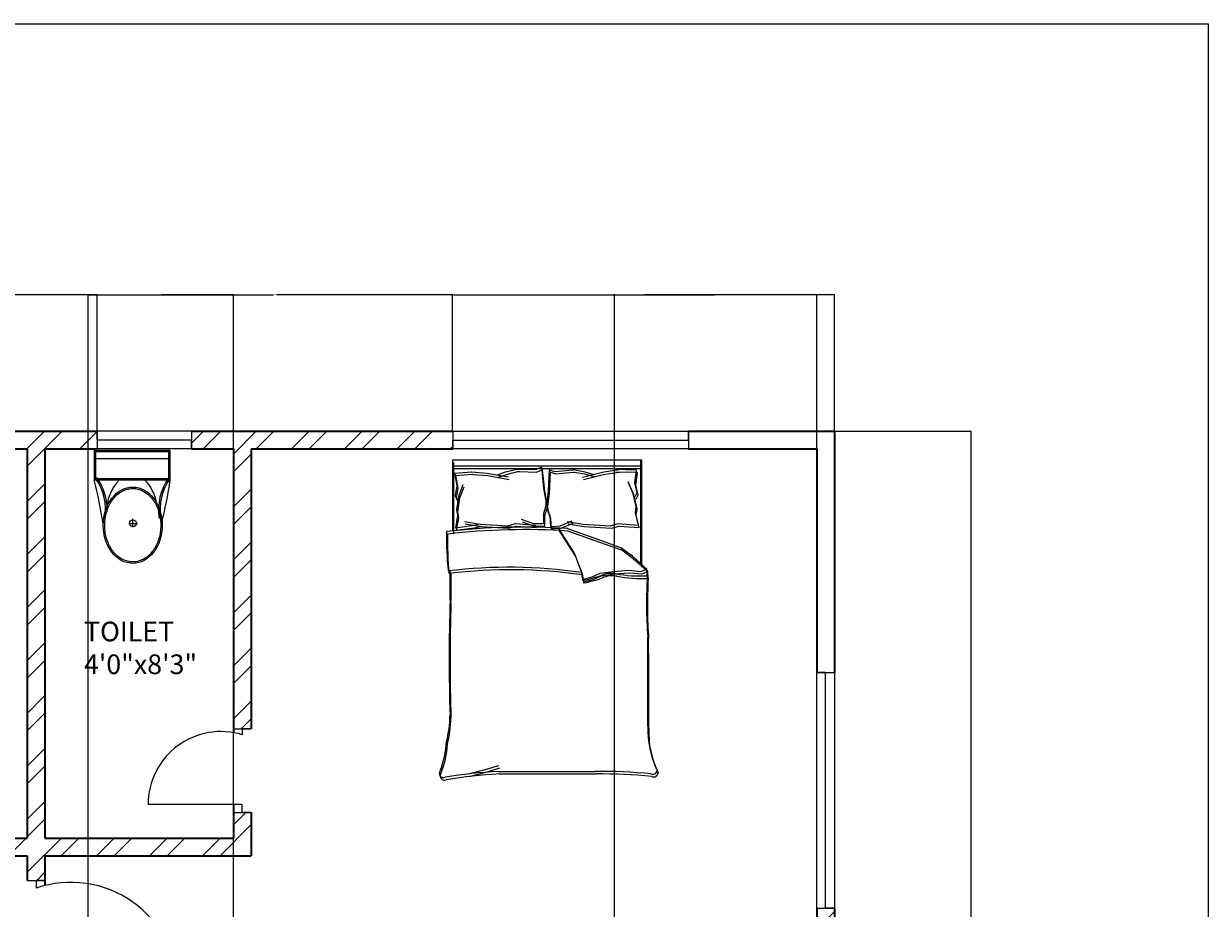
# Model space of a CAD drawing. Units: inches. Extents: x 1965 to 2673, y 1802 to 2669.
# Tile 16 of 16: x 2372 to 2673, y 2444 to 2669. Entities that reach past the tile are written whole.
import ezdxf

# ---------------------------------------------------------------- set-up
doc = ezdxf.new("R2010")
doc.units = ezdxf.units.IN
for name, color, linetype, lineweight in [('A-ANNO-DIMS', 2, 'Continuous', 18), ('A-ANNO-TTLB', 7, 'Continuous', 25), ('A-AREA-IDEN', 7, 'Continuous', 18), ('A-DOOR', 11, 'Continuous', 18), ('A-FLOR-FIXT', 9, 'Continuous', 18), ('A-FURN', 8, 'Continuous', 13), ('A-GLAZ', 181, 'Continuous', 18), ('A-WALL', 7, 'Continuous', 35), ('A-WALL-PATT', 252, 'Continuous', 13)]:
    doc.layers.add(name, color=color, linetype=linetype, lineweight=lineweight)
doc.styles.get("Standard").update_dxf_attribs({"font": 'arial.ttf'})
doc.dimstyles.get("Standard").update_dxf_attribs({"dimtxt": 0.18, "dimasz": 0.18, "dimexe": 0.18, "dimexo": 0.0625, "dimgap": 0.09, "dimtad": 0, "dimtih": 1, "dimtoh": 1, "dimdec": 4, "dimzin": 0, "dimdsep": 46, "dimtxsty": 'Standard', "dimcen": 0.09, "dimadec": 0, "dimazin": 0, "dimtfac": 1, "dimtdec": 4, "dimtofl": 0, "dimtmove": 0, "dimatfit": 3, "dimfxl": 1, "dimtolj": 1, "dimtzin": 0, "dimarcsym": 0})

# ---------------------------------------------------------------- blocks, each defined once
blk = doc.blocks.new('A$C31115884')
for p, q in [((283.1, 497.7), (223.4, 497.7)), ((257.5, 466.4), (257.5, 523.2)), ((0, 200), (0, 0)), ((520, 200), (0, 200)), ((10, 190), (10, 10)), ((510, 190), (10, 190)), ((510, 10), (510, 190)), ((520, 0), (520, 200)), ((510, 54.5), (0, 54.5)), ((10, 10), (510, 10)), ((0, 0), (520, 0))]:
    blk.add_line(p, q)
blk.add_circle((255.6, 496.4), 23.6)
for centre, radius, start, end in [((2777.7, -204.6), 2807, 165.4549, 171.71327), ((3237, 905), 2807, 188.28673, 194.5451), ((-294.5, 403.3), 364.7, 324.20913, 9.34987), ((-294.5, 403.3), 374.7, 324.20913, 9.34987), ((139.5, 406.2), 293.5, 315.84364, 2.65635), ((805.8, 403.3), 374.7, 179.20365, 215.79087), ((805.8, 403.3), 364.7, 170.65013, 215.79087), ((383.6, 406.2), 293.5, 190.27735, 224.15636)]:
    blk.add_arc(centre, radius, start, end)
blk.add_ellipse((256.2, 509.9), major_axis=(0, -260.7), ratio=0.772727)
blk.add_open_spline([(256.2, 259.2), (263.1, 259.2), (270, 259.7), (287.8, 262.3), (298.7, 265.1), (319.9, 273.1), (330.2, 278.4), (350.1, 291.1), (359.7, 298.7), (377.7, 315.9), (386.2, 325.5), (401.7, 346.6), (408.8, 358.1), (421.3, 382.5), (426.8, 395.5), (435.9, 422.4), (439.5, 436.4), (444.8, 465.1), (446.5, 479.7), (447.9, 509.2), (447.6, 524), (445, 553.3), (442.7, 567.8), (436.3, 596), (432.1, 609.7), (421.9, 636), (416, 648.6), (402.5, 672.1), (395, 683), (378.6, 703), (369.8, 712.1), (351.1, 728), (341.3, 734.8), (320.9, 746.2), (310.4, 750.7), (288.9, 757.3), (278, 759.4), (256, 761), (245, 760.6), (223.1, 757.2), (212.3, 754.3), (191.1, 746.1), (180.8, 740.7), (160.9, 727.8), (151.4, 720.1), (133.5, 702.7), (125.1, 693), (109.6, 671.7), (102.6, 660.2), (90.2, 635.7), (84.9, 622.7), (76, 595.6), (72.4, 581.6), (67.2, 552.9), (65.6, 538.2), (64.4, 508.8), (64.8, 494), (67.5, 464.7), (69.9, 450.2), (76.6, 422), (80.8, 408.3), (91.1, 382.2), (97.2, 369.7), (110.8, 346.3), (118.4, 335.4), (134.8, 315.6), (143.7, 306.7), (162.4, 290.9), (172.3, 284.2), (192.8, 273), (203.3, 268.6), (224.8, 262.2), (235.8, 260.2), (249.9, 259.3), (253, 259.2), (256.2, 259.2)], degree=3, knots=[0, 0, 0, 0, 0.110105, 0.110105, 0.285049, 0.285049, 0.459994, 0.459994, 0.634938, 0.634938, 0.809882, 0.809882, 0.984827, 0.984827, 1.159771, 1.159771, 1.334715, 1.334715, 1.50966, 1.50966, 1.684604, 1.684604, 1.859549, 1.859549, 2.034493, 2.034493, 2.209437, 2.209437, 2.384382, 2.384382, 2.559326, 2.559326, 2.73427, 2.73427, 2.909215, 2.909215, 3.084159, 3.084159, 3.259103, 3.259103, 3.434048, 3.434048, 3.608992, 3.608992, 3.783936, 3.783936, 3.958881, 3.958881, 4.133825, 4.133825, 4.30877, 4.30877, 4.483714, 4.483714, 4.658658, 4.658658, 4.833603, 4.833603, 5.008547, 5.008547, 5.183491, 5.183491, 5.358436, 5.358436, 5.53338, 5.53338, 5.708324, 5.708324, 5.883269, 5.883269, 6.058213, 6.058213, 6.233158, 6.233158, 6.283185, 6.283185, 6.283185, 6.283185])
blk = doc.blocks.new('BED-DOUBLE')
for p, q in [((3.47, 63.33), (3.47, 81.44)), ((3.47, 63.33), (3.47, 81.44)), ((3.47, 81.44), (51.49, 81.44)), ((51.26, 81.44), (51.26, 54.83)), ((51.26, 81.44), (51.26, 54.83)), ((51.49, 81.44), (51.49, 80.8)), ((3.47, 79.91), (51.26, 79.91)), ((3.47, 79.91), (51.26, 79.91)), ((3.7, 62.69), (3.7, 80.8)), ((3.7, 62.69), (3.7, 80.8)), ((3.7, 79.27), (51.49, 79.27)), ((3.7, 79.27), (51.49, 79.27)), ((3.89, 78.1), (8.17, 78.43)), ((3.89, 78.1), (8.17, 78.43)), ((8.17, 78.43), (8.28, 78.41)), ((8.17, 78.43), (8.28, 78.41)), ((8.28, 78.41), (12.1, 78.12)), ((8.28, 78.41), (12.1, 78.12)), ((14.85, 77.69), (16.87, 78.41)), ((14.85, 77.69), (16.87, 78.41)), ((16.87, 78.41), (19.76, 79.14)), ((16.87, 78.41), (19.76, 79.14)), ((17.1, 77.77), (19.99, 78.5)), ((17.1, 77.77), (19.99, 78.5)), ((19.76, 79.14), (20.09, 79.14)), ((19.76, 79.14), (20.09, 79.14)), ((19.99, 78.5), (20.31, 78.5)), ((19.99, 78.5), (20.31, 78.5)), ((20.09, 79.14), (24.53, 78.99)), ((20.09, 79.14), (24.53, 78.99)), ((20.31, 78.5), (24.76, 78.35)), ((20.31, 78.5), (24.76, 78.35)), ((24.53, 78.99), (25.98, 79.57)), ((24.53, 78.99), (25.98, 79.57)), ((24.76, 78.35), (26.21, 78.93)), ((24.76, 78.35), (26.21, 78.93)), ((25.98, 79.57), (26.56, 74.22)), ((25.98, 79.57), (26.56, 74.22)), ((26.21, 78.93), (26.78, 73.58)), ((26.21, 78.93), (26.78, 73.58)), ((27.97, 78.95), (27.73, 73.57)), ((27.97, 78.95), (27.73, 73.57)), ((29.45, 78.46), (27.97, 78.95)), ((29.45, 78.46), (27.97, 78.95)), ((33.88, 78.88), (29.45, 78.46)), ((33.88, 78.88), (29.45, 78.46)), ((34.2, 78.9), (33.88, 78.88)), ((34.2, 78.9), (33.88, 78.88)), ((37.13, 78.36), (34.2, 78.9)), ((37.13, 78.36), (34.2, 78.9)), ((45.71, 78.9), (41.91, 78.37)), ((45.71, 78.9), (41.91, 78.37)), ((50.11, 78.88), (44.7, 78.98)), ((44.7, 78.98), (45.71, 78.9)), ((50.11, 78.88), (44.7, 78.98)), ((44.7, 78.98), (45.71, 78.9)), ((50.11, 78.88), (49.73, 75.67)), ((50.11, 78.88), (49.73, 75.67)), ((51.49, 80.8), (51.49, 54.19)), ((51.49, 80.8), (51.49, 54.19)), ((3.89, 78.12), (4.47, 74.94)), ((3.89, 78.12), (4.47, 74.94)), ((4.12, 77.46), (8.4, 77.79)), ((4.12, 77.46), (8.4, 77.79)), ((4.12, 77.49), (4.7, 74.3)), ((4.12, 77.49), (4.7, 74.3)), ((8.4, 77.79), (8.51, 77.77)), ((8.4, 77.79), (8.51, 77.77)), ((8.51, 77.77), (12.33, 77.49)), ((8.51, 77.77), (12.33, 77.49)), ((12.1, 78.12), (17.6, 77.11)), ((12.1, 78.12), (17.6, 77.11)), ((12.33, 77.49), (17.82, 76.47)), ((12.33, 77.49), (17.82, 76.47)), ((15.08, 77.05), (17.1, 77.77)), ((15.08, 77.05), (17.1, 77.77)), ((28.2, 78.31), (27.96, 72.93)), ((28.2, 78.31), (27.96, 72.93)), ((29.68, 77.82), (28.2, 78.31)), ((29.68, 77.82), (28.2, 78.31)), ((34.11, 78.24), (29.68, 77.82)), ((34.11, 78.24), (29.68, 77.82)), ((34.43, 78.26), (34.11, 78.24)), ((34.43, 78.26), (34.11, 78.24)), ((37.36, 77.72), (34.43, 78.26)), ((37.36, 77.72), (34.43, 78.26)), ((41.91, 78.37), (36.49, 77.02)), ((41.91, 78.37), (36.49, 77.02)), ((42.14, 77.73), (36.72, 76.38)), ((42.14, 77.73), (36.72, 76.38)), ((39.2, 77.77), (37.13, 78.36)), ((39.19, 77.77), (37.13, 78.36)), ((39.42, 77.13), (37.36, 77.72)), ((39.42, 77.13), (37.36, 77.72)), ((45.94, 78.26), (42.14, 77.73)), ((45.94, 78.26), (42.14, 77.73)), ((50.34, 78.24), (44.93, 78.34)), ((44.93, 78.34), (45.94, 78.26)), ((50.34, 78.24), (44.93, 78.34)), ((44.93, 78.34), (45.94, 78.26)), ((49.3, 73.18), (48.12, 75.86)), ((49.3, 73.18), (48.12, 75.86)), ((49.73, 75.67), (50.32, 73.1)), ((49.73, 75.67), (50.32, 73.1)), ((50.34, 78.24), (49.96, 75.03)), ((50.34, 78.24), (49.96, 75.03)), ((4.47, 74.94), (4.03, 72.34)), ((4.47, 74.94), (4.03, 72.34)), ((4.7, 74.3), (4.26, 71.7)), ((4.7, 74.3), (4.26, 71.7)), ((4.47, 68.87), (5.05, 72.49)), ((4.47, 68.87), (5.05, 72.49)), ((5.05, 72.49), (6.06, 75.23)), ((5.05, 72.49), (6.06, 75.23)), ((5.27, 71.85), (6.29, 74.59)), ((5.27, 71.85), (6.29, 74.59)), ((26.56, 74.22), (27.13, 71.04)), ((26.56, 74.22), (27.13, 71.04)), ((26.78, 73.58), (27.36, 70.4)), ((26.78, 73.58), (27.36, 70.4)), ((27.73, 73.57), (27.35, 70.36)), ((27.73, 73.57), (27.35, 70.36)), ((27.96, 72.93), (27.58, 69.72)), ((27.96, 72.93), (27.58, 69.72)), ((49.53, 72.54), (48.35, 75.22)), ((49.53, 72.54), (48.35, 75.22)), ((50.11, 69.61), (49.3, 73.18)), ((50.11, 69.61), (49.3, 73.18)), ((50.34, 68.97), (49.53, 72.54)), ((50.34, 68.97), (49.53, 72.54)), ((50.32, 73.1), (49.81, 72.06)), ((50.32, 73.1), (49.81, 72.06)), ((49.96, 75.03), (50.55, 72.46)), ((49.96, 75.03), (50.55, 72.46)), ((50.55, 72.46), (50.04, 71.42)), ((50.55, 72.46), (50.04, 71.42)), ((4.03, 72.34), (4.61, 71.33)), ((4.03, 72.34), (4.61, 71.33)), ((4.26, 71.7), (4.84, 70.69)), ((4.26, 71.7), (4.84, 70.69)), ((4.7, 68.23), (5.27, 71.85)), ((4.7, 68.23), (5.27, 71.85)), ((27.13, 69.74), (26.56, 67.86)), ((27.13, 69.74), (26.56, 67.86)), ((27.13, 71.04), (27.13, 69.74)), ((27.13, 71.04), (27.13, 69.74)), ((27.35, 70.36), (27.43, 69.06)), ((27.35, 70.36), (27.43, 69.06)), ((27.36, 70.4), (27.36, 69.1)), ((27.36, 70.4), (27.36, 69.1)), ((27.58, 69.72), (27.66, 68.42)), ((27.58, 69.72), (27.66, 68.42)), ((49.92, 68.01), (50.11, 69.61)), ((49.92, 68.01), (50.11, 69.61)), ((4.18, 64.1), (4.76, 67.28)), ((4.18, 64.1), (4.76, 67.28)), ((4.41, 63.46), (4.99, 66.64)), ((4.41, 63.46), (4.99, 66.64)), ((4.76, 67.28), (4.47, 68.87)), ((4.76, 67.28), (4.47, 68.87)), ((4.99, 66.64), (4.7, 68.23)), ((4.99, 66.64), (4.7, 68.23)), ((26.56, 67.86), (26.56, 65.18)), ((26.56, 67.86), (26.56, 65.18)), ((27.36, 69.1), (26.78, 67.22)), ((27.36, 69.1), (26.78, 67.22)), ((26.78, 67.22), (26.78, 64.54)), ((26.78, 67.22), (26.78, 64.54)), ((27.43, 69.06), (28.13, 67.22)), ((27.43, 69.06), (28.13, 67.22)), ((27.66, 68.42), (28.35, 66.58)), ((27.66, 68.42), (28.35, 66.58)), ((28.13, 67.22), (28.29, 64.55)), ((28.13, 67.22), (28.29, 64.55)), ((28.35, 66.58), (28.52, 63.91)), ((28.35, 66.58), (28.52, 63.91)), ((50.69, 64.87), (49.92, 68.01)), ((50.69, 64.87), (49.92, 68.01)), ((50.15, 67.37), (50.34, 68.97)), ((50.15, 67.37), (50.34, 68.97)), ((50.92, 64.23), (50.15, 67.37)), ((50.92, 64.23), (50.15, 67.37)), ((9.28, 64.82), (4.18, 64.1)), ((9.28, 64.82), (4.18, 64.1)), ((9.5, 64.18), (4.41, 63.46)), ((9.5, 64.18), (4.41, 63.46)), ((6.38, 65.81), (10.41, 65.15)), ((6.38, 65.81), (10.41, 65.15)), ((6.6, 65.17), (10.64, 64.51)), ((6.61, 65.17), (10.64, 64.51)), ((10.41, 65.15), (9.28, 64.82)), ((10.41, 65.15), (9.28, 64.82)), ((10.64, 64.51), (9.5, 64.18)), ((10.64, 64.51), (9.5, 64.18)), ((10.41, 65.15), (17.42, 64.71)), ((10.41, 65.15), (17.42, 64.71)), ((10.64, 64.51), (17.65, 64.08)), ((10.64, 64.51), (17.65, 64.08)), ((17.42, 64.71), (19.38, 65.27)), ((17.42, 64.71), (19.38, 65.27)), ((17.65, 64.08), (19.61, 64.63)), ((17.65, 64.08), (19.61, 64.63)), ((19.38, 65.27), (24.51, 64.87)), ((19.38, 65.27), (24.51, 64.87)), ((19.61, 64.63), (24.74, 64.23)), ((19.61, 64.63), (24.74, 64.23)), ((24.1, 65.18), (20.95, 66.27)), ((24.1, 65.18), (20.95, 66.27)), ((24.33, 64.54), (21.18, 65.63)), ((24.33, 64.54), (21.18, 65.63)), ((26.56, 65.18), (24.1, 65.18)), ((26.56, 65.18), (24.1, 65.18)), ((26.78, 64.54), (24.33, 64.54)), ((26.78, 64.54), (24.33, 64.54)), ((28.29, 64.55), (30.75, 64.7)), ((28.29, 64.55), (30.75, 64.7)), ((28.52, 63.91), (30.97, 64.06)), ((28.52, 63.91), (30.97, 64.06)), ((30.25, 64.06), (34.44, 57.56)), ((30.25, 64.06), (34.44, 57.56)), ((30.48, 63.42), (34.67, 56.92)), ((30.48, 63.42), (34.67, 56.92)), ((30.75, 64.7), (33.82, 65.99)), ((30.75, 64.7), (33.82, 65.99)), ((30.97, 64.06), (34.04, 65.35)), ((30.97, 64.06), (34.04, 65.35)), ((40.64, 61.12), (32.3, 64.06)), ((40.64, 61.12), (32.3, 64.06)), ((40.87, 60.48), (32.53, 63.42)), ((40.87, 60.48), (32.53, 63.42)), ((32.56, 65.81), (36.59, 65.15)), ((32.56, 65.81), (36.59, 65.15)), ((32.79, 65.17), (36.82, 64.51)), ((32.79, 65.17), (36.82, 64.51)), ((36.59, 65.15), (43.6, 64.71)), ((36.59, 65.15), (43.6, 64.71)), ((36.82, 64.51), (43.83, 64.08)), ((36.82, 64.51), (43.83, 64.08)), ((43.6, 64.71), (45.56, 65.27)), ((43.6, 64.71), (45.56, 65.27)), ((43.83, 64.08), (45.79, 64.63)), ((43.83, 64.08), (45.79, 64.63)), ((45.56, 65.27), (50.69, 64.87)), ((45.56, 65.27), (50.69, 64.87)), ((45.79, 64.63), (50.92, 64.23)), ((45.79, 64.63), (50.92, 64.23)), ((46.21, 59.11), (40.64, 61.12)), ((46.21, 59.11), (40.64, 61.12)), ((46.44, 58.47), (40.87, 60.48)), ((46.44, 58.47), (40.87, 60.48)), ((34.44, 57.56), (36.15, 53.08)), ((34.44, 57.56), (36.15, 53.08)), ((49.16, 56.95), (46.21, 59.11)), ((49.16, 56.95), (46.21, 59.11)), ((49.39, 56.31), (46.44, 58.47)), ((49.39, 56.31), (46.44, 58.47)), ((34.67, 56.92), (36.38, 52.44)), ((34.67, 56.92), (36.38, 52.44)), ((52.86, 53.69), (49.16, 56.95)), ((52.86, 53.69), (49.16, 56.95)), ((53.09, 53.06), (49.39, 56.31)), ((53.09, 53.06), (49.39, 56.31)), ((36.15, 53.08), (36.46, 51.06)), ((36.15, 53.08), (36.46, 51.06)), ((36.38, 52.44), (36.69, 50.42)), ((36.38, 52.44), (36.69, 50.42)), ((36.46, 51.06), (38.94, 51.68)), ((36.46, 51.06), (38.94, 51.68)), ((38.94, 51.68), (40.95, 52.61)), ((38.94, 51.68), (40.95, 52.61)), ((39.16, 51.04), (41.18, 51.97)), ((39.16, 51.04), (41.18, 51.97)), ((40.95, 52.61), (44.36, 53.08)), ((40.95, 52.61), (44.36, 53.08)), ((41.18, 51.97), (44.58, 52.44)), ((41.18, 51.97), (44.58, 52.44)), ((44.36, 53.08), (48.23, 53.39)), ((44.36, 53.08), (48.23, 53.39)), ((44.58, 52.44), (48.46, 52.75)), ((44.58, 52.44), (48.46, 52.75)), ((48.23, 53.39), (51.33, 53.08)), ((48.23, 53.39), (51.33, 53.08)), ((48.46, 52.75), (51.55, 52.44)), ((48.46, 52.75), (51.55, 52.44)), ((51.33, 53.08), (52.86, 53.69)), ((51.33, 53.08), (52.86, 53.69)), ((51.55, 52.44), (53.09, 53.06)), ((51.55, 52.44), (53.09, 53.06)), ((52.94, 51.95), (52.86, 53.69, 3.87)), ((52.94, 51.95), (52.86, 53.69, 3.87)), ((53.17, 51.31), (53.09, 53.06, 3.87)), ((53.17, 51.31), (53.09, 53.06, 3.87)), ((36.69, 50.42), (39.16, 51.04)), ((36.69, 50.42), (39.16, 51.04)), ((15.06, 2.2), (39.67, 2.2)), ((15.06, 2.2), (39.67, 2.2)), ((15.29, 1.56), (39.9, 1.56)), ((15.29, 1.56), (39.9, 1.56))]:
    blk.add_line(p, q)
for centre, radius, start, end in [((21.35, -100.61), 164.97, 86.0865, 96.7821), ((21.35, -100.61), 164.97, 86.0865, 96.7821), ((21.58, -101.25), 164.97, 86.0865, 96.7821), ((21.58, -101.25), 164.97, 86.0865, 96.7821), ((85.16, 61.34), 83.31, 178.7218, 185.604), ((85.16, 61.34), 83.31, 178.7218, 185.604), ((85.39, 60.71), 83.31, 178.7218, 185.604), ((85.38, 60.71), 83.31, 178.7218, 185.604), ((17.75, -74.88), 129.02, 81.7845, 96.9006), ((17.75, -74.88), 129.02, 81.7845, 96.9006), ((17.98, -75.51), 129.02, 81.7845, 96.9006), ((17.98, -75.51), 129.02, 81.7845, 96.9006), ((-167.31, 50.27), 170.11, 358.4762, 1.0082), ((-167.31, 50.27), 170.11, 358.4762, 1.0082), ((-167.08, 49.63), 170.11, 358.4762, 1.0082), ((-167.08, 49.63), 170.11, 358.4762, 1.0082), ((31.15, 79.96), 29.65, 280.6617, 289.8806), ((31.15, 79.96), 29.65, 280.6617, 289.8806), ((31.38, 79.32), 29.65, 280.6617, 289.8806), ((31.38, 79.32), 29.65, 280.6617, 289.8806), ((43.74, 46.37), 6.22, 78.6608, 113.7384), ((43.74, 46.37), 6.22, 78.6608, 113.7384), ((43.97, 45.74), 6.22, 78.6608, 113.7384), ((43.97, 45.74), 6.22, 78.6608, 113.7384), ((51.32, 88.1), 36.18, 259.8763, 272.5657), ((51.32, 88.1), 36.18, 259.8763, 272.5657), ((51.55, 87.46), 36.18, 259.8763, 272.5657), ((51.55, 87.46), 36.18, 259.8763, 272.5657), ((182.26, 45.13), 129.5, 176.9791, 183.8365), ((182.26, 45.13), 129.5, 176.9791, 183.8365), ((182.49, 44.49), 129.5, 176.9791, 183.8365), ((182.49, 44.49), 129.5, 176.9791, 183.8365), ((36.63, 51), 0.185, 160.2464, 271.1377), ((36.63, 51), 0.185, 160.2464, 271.1377), ((36.86, 50.36), 0.185, 160.2464, 271.1377), ((36.86, 50.36), 0.185, 160.2464, 271.1377), ((484.82, 30.83), 482.31, 178.2277, 181.7185), ((484.82, 30.83), 482.31, 178.2277, 181.7185), ((485.05, 30.19), 482.31, 178.2277, 181.7185), ((485.05, 30.19), 482.31, 178.2277, 181.7185), ((-4508.75, 13.62), 4561.86, 0.00217, 0.28689), ((-4508.75, 13.62), 4561.86, 0.00217, 0.28689), ((-4508.52, 12.98), 4561.86, 0.00217, 0.28689), ((-4508.52, 12.98), 4561.86, 0.00217, 0.28689), ((-26.9, 16.93), 29.63, 346.0648, 358.9113), ((-26.9, 16.93), 29.63, 346.0648, 358.9113), ((-26.68, 16.29), 29.63, 346.0648, 358.9113), ((-26.68, 16.29), 29.63, 346.0648, 358.9113), ((76.15, 12.77), 23.07, 177.4714, 206.4681), ((76.15, 12.77), 23.07, 177.4714, 206.4681), ((76.38, 12.14), 23.07, 177.4714, 206.4681), ((76.38, 12.14), 23.07, 177.4714, 206.4681), ((-21.66, 11.17), 23.56, 337.9751, 356.652), ((-21.66, 11.17), 23.56, 337.9751, 356.652), ((-21.44, 10.53), 23.56, 337.9751, 356.652), ((-21.44, 10.53), 23.56, 337.9751, 356.652), ((-17.23, 105.15), 106.46, 283.3832, 287.7053), ((-17.23, 105.15), 106.46, 283.3832, 287.7053), ((-17, 104.51), 106.46, 283.3832, 287.7053), ((-17, 104.51), 106.46, 283.3832, 287.7053), ((1.08, 1.72), 1.09, 146.1736, 293.4781), ((1.08, 1.72), 1.09, 146.1736, 293.4781), ((1.31, 1.08), 1.09, 146.1736, 293.4781), ((1.31, 1.08), 1.09, 146.1736, 293.4781), ((21.42, -119.4), 121.76, 92.9958, 99.4091), ((21.42, -119.4), 121.76, 92.9958, 99.4091), ((21.65, -120.04), 121.76, 92.9958, 99.4091), ((21.65, -120.04), 121.76, 92.9958, 99.4091), ((41.15, -130.84), 133.04, 84.4998, 90.6351), ((41.15, -130.84), 133.04, 84.4998, 90.6351), ((41.38, -131.48), 133.04, 84.4998, 90.6351), ((41.37, -131.48), 133.04, 84.4998, 90.6351), ((54.4, 2.57), 1.1, 242.6588, 356.02), ((54.4, 2.57), 1.1, 242.6588, 356.02), ((54.63, 1.93), 1.1, 242.6588, 356.02), ((54.63, 1.93), 1.1, 242.6588, 356.02)]:
    blk.add_arc(centre, radius, start, end)
blk = doc.blocks.new('WIN-60IN')
for p, q in [((0, 4.5), (0, 0)), ((0, 4.5), (60, 4.5)), ((60, 2.25), (60, 4.5)), ((60, 4.5), (60, 0)), ((0, 0), (0, 2.25)), ((0, 2.25), (60, 2.25)), ((60, 0), (0, 0))]:
    blk.add_line(p, q)
blk = doc.blocks.new('WIN-24IN')
for p, q in [((0, 24), (4.5, 24)), ((0, 24), (0, 0)), ((4.5, 24), (2.25, 24)), ((2.25, 24), (2.25, 0)), ((4.5, 24), (4.5, 0)), ((2.25, 0), (0, 0)), ((0, 0), (4.5, 0))]:
    blk.add_line(p, q)
blk = doc.blocks.new('*D26')
at = {"layer": 'A-ANNO-DIMS', "color": 0, "lineweight": -2, "transparency": 16777216}
for p, q in [((2578.16, 2565.59), (2613, 2565.59)), ((2612.82, 2565.41), (2612.82, 2248.77)), ((2612.82, 1931.77), (2612.82, 2248.41)), ((2578.16, 1931.59), (2613, 1931.59))]:
    blk.add_line(p, q, dxfattribs=at)
at = {"layer": 'A-ANNO-DIMS', "color": 0, "transparency": 16777216}
for points in [[(2612.79, 2565.41), (2612.85, 2565.41), (2612.82, 2565.59)], [(2612.79, 1931.77), (2612.85, 1931.77), (2612.82, 1931.59)]]:
    blk.add_solid(points, dxfattribs=at)
at = {"layer": 'Defpoints', "color": 0, "transparency": 16777216}
for p in [(2578.09, 2565.59), (2612.82, 2565.59), (2578.09, 1931.59)]:
    blk.add_point(p, dxfattribs=at)
at = {"layer": 'A-ANNO-DIMS', "color": 0, "transparency": 16777216, "insert": (2612.82, 2248.59), "char_height": 0.18, "attachment_point": 5}
blk.add_mtext('\\A1;634', dxfattribs=at)
blk = doc.blocks.new('*D30')
at = {"layer": 'A-ANNO-DIMS', "color": 0, "lineweight": -2, "transparency": 16777216}
for p, q in [((2285.97, 2565.65), (2285.97, 2600.5)), ((2286.15, 2600.32), (2337.74, 2600.32)), ((2390.24, 2600.32), (2338.65, 2600.32)), ((2390.42, 2565.65), (2390.42, 2600.5))]:
    blk.add_line(p, q, dxfattribs=at)
at = {"layer": 'A-ANNO-DIMS', "color": 0, "transparency": 16777216}
for points in [[(2286.15, 2600.35), (2286.15, 2600.29), (2285.97, 2600.32)], [(2390.24, 2600.35), (2390.24, 2600.29), (2390.42, 2600.32)]]:
    blk.add_solid(points, dxfattribs=at)
at = {"layer": 'Defpoints', "color": 0, "transparency": 16777216}
for p in [(2390.42, 2600.32), (2285.97, 2565.59), (2390.42, 2565.59)]:
    blk.add_point(p, dxfattribs=at)
at = {"layer": 'A-ANNO-DIMS', "color": 0, "transparency": 16777216, "insert": (2338.2, 2600.32), "char_height": 0.18, "attachment_point": 5}
blk.add_mtext('\\A1;104.44', dxfattribs=at)
blk = doc.blocks.new('*D31')
at = {"layer": 'A-ANNO-DIMS', "color": 0, "lineweight": -2, "transparency": 16777216}
for p, q in [((2390.42, 2565.65), (2390.42, 2600.5)), ((2390.6, 2600.32), (2435.26, 2600.32)), ((2480.71, 2600.32), (2436.05, 2600.32)), ((2480.89, 2565.65), (2480.89, 2600.5))]:
    blk.add_line(p, q, dxfattribs=at)
at = {"layer": 'A-ANNO-DIMS', "color": 0, "transparency": 16777216}
for points in [[(2390.6, 2600.35), (2390.6, 2600.29), (2390.42, 2600.32)], [(2480.71, 2600.35), (2480.71, 2600.29), (2480.89, 2600.32)]]:
    blk.add_solid(points, dxfattribs=at)
at = {"layer": 'Defpoints', "color": 0, "transparency": 16777216}
for p in [(2480.89, 2600.32), (2390.42, 2565.59), (2480.89, 2565.59)]:
    blk.add_point(p, dxfattribs=at)
at = {"layer": 'A-ANNO-DIMS', "color": 0, "transparency": 16777216, "insert": (2435.66, 2600.32), "char_height": 0.18, "attachment_point": 5}
blk.add_mtext('\\A1;90.48', dxfattribs=at)
blk = doc.blocks.new('*D32')
at = {"layer": 'A-ANNO-DIMS', "color": 0, "lineweight": -2, "transparency": 16777216}
for p, q in [((2480.89, 2565.65), (2480.89, 2600.5)), ((2481.07, 2600.32), (2529.17, 2600.32)), ((2577.91, 2600.32), (2529.82, 2600.32)), ((2578.09, 2565.65), (2578.09, 2600.5))]:
    blk.add_line(p, q, dxfattribs=at)
at = {"layer": 'A-ANNO-DIMS', "color": 0, "transparency": 16777216}
for points in [[(2481.07, 2600.35), (2481.07, 2600.29), (2480.89, 2600.32)], [(2577.91, 2600.35), (2577.91, 2600.29), (2578.09, 2600.32)]]:
    blk.add_solid(points, dxfattribs=at)
at = {"layer": 'Defpoints', "color": 0, "transparency": 16777216}
for p in [(2578.09, 2600.32), (2480.89, 2565.59), (2578.09, 2565.59)]:
    blk.add_point(p, dxfattribs=at)
at = {"layer": 'A-ANNO-DIMS', "color": 0, "transparency": 16777216, "insert": (2529.49, 2600.32), "char_height": 0.18, "attachment_point": 5}
blk.add_mtext('\\A1;97.2', dxfattribs=at)
blk = doc.blocks.new('*D44')
at = {"layer": 'A-ANNO-DIMS', "color": 0, "lineweight": -2, "transparency": 16777216}
for p, q in [((2522.13, 1936.15), (2522.13, 2600.5)), ((2522.31, 2600.32), (2547.47, 2600.32)), ((2573.41, 2600.32), (2548.26, 2600.32)), ((2573.59, 1936.15), (2573.59, 2600.5))]:
    blk.add_line(p, q, dxfattribs=at)
at = {"layer": 'A-ANNO-DIMS', "color": 0, "transparency": 16777216}
for points in [[(2522.31, 2600.35), (2522.31, 2600.29), (2522.13, 2600.32)], [(2573.41, 2600.35), (2573.41, 2600.29), (2573.59, 2600.32)]]:
    blk.add_solid(points, dxfattribs=at)
at = {"layer": 'Defpoints', "color": 0, "transparency": 16777216}
for p in [(2573.59, 2600.32), (2522.13, 1936.09), (2573.59, 1936.09)]:
    blk.add_point(p, dxfattribs=at)
at = {"layer": 'A-ANNO-DIMS', "color": 0, "transparency": 16777216, "insert": (2547.86, 2600.32), "char_height": 0.18, "attachment_point": 5}
blk.add_mtext('\\A1;51.46', dxfattribs=at)
blk = doc.blocks.new('*D50')
at = {"layer": 'A-ANNO-DIMS', "color": 0, "lineweight": -2, "transparency": 16777216}
for p, q in [((2388.09, 2116.15), (2388.09, 2600.5)), ((2388.27, 2600.32), (2406.37, 2600.32)), ((2424.91, 2600.32), (2406.81, 2600.32)), ((2425.09, 2116.15), (2425.09, 2600.5))]:
    blk.add_line(p, q, dxfattribs=at)
at = {"layer": 'A-ANNO-DIMS', "color": 0, "transparency": 16777216}
for points in [[(2388.27, 2600.35), (2388.27, 2600.29), (2388.09, 2600.32)], [(2424.91, 2600.35), (2424.91, 2600.29), (2425.09, 2600.32)]]:
    blk.add_solid(points, dxfattribs=at)
at = {"layer": 'Defpoints', "color": 0, "transparency": 16777216}
for p in [(2425.09, 2600.32), (2388.09, 2116.09), (2425.09, 2116.09)]:
    blk.add_point(p, dxfattribs=at)
at = {"layer": 'A-ANNO-DIMS', "color": 0, "transparency": 16777216, "insert": (2406.59, 2600.32), "char_height": 0.18, "attachment_point": 5}
blk.add_mtext('\\A1;37', dxfattribs=at)

msp = doc.modelspace()

# ---------------------------------------------------------------- hatches: boundary and pattern name
at = {"layer": 'A-WALL-PATT'}
h = msp.add_hatch(dxfattribs=at)
h.set_pattern_fill('ANSI32', color=256)
h.paths.add_polyline_path([(2051.5927, 2561.0914), (2076.7559, 2561.0914), (2076.7559, 2563.3414), (2076.7559, 2565.5914), (2047.0927, 2565.5914), (2047.0927, 2518.3824), (2051.5927, 2518.3824)])
h.paths.add_polyline_path([(2051.5927, 2458.3824), (2049.3427, 2458.3824), (2047.0927, 2458.3824), (2047.0927, 2412.5914), (2248.0927, 2412.5914), (2248.0927, 2268.5914), (2252.5927, 2268.5914), (2252.5927, 2412.5914), (2252.5927, 2421.0404), (2250.3427, 2421.0404), (2248.0927, 2421.0404), (2248.0927, 2417.0914), (2051.5927, 2417.0914)])
h.paths.add_polyline_path([(2211.4933, 2268.5914), (2104.0927, 2268.5914), (2104.0927, 2272.4654), (2101.8427, 2272.4654), (2099.5927, 2272.4654), (2099.5927, 2268.5914), (2051.5927, 2268.5914), (2051.5927, 2264.0914), (2147.5927, 2264.0914), (2147.5927, 2259.8893), (2152.0927, 2259.8893), (2152.0927, 2264.0914), (2211.4933, 2264.0914), (2211.4933, 2266.3414)])
h.paths.add_polyline_path([(2104.0927, 2376.0914), (2099.5927, 2376.0914), (2047.0927, 2376.0914), (2047.0927, 2333.0682), (2051.5927, 2333.0682), (2051.5927, 2371.5914), (2099.5927, 2371.5914), (2099.5927, 2293.6123), (2104.0927, 2293.6123)], flags=17)
h.paths.add_polyline_path([(2051.5927, 2309.0682), (2047.0927, 2309.0682), (2047.0927, 2233.5821), (2051.5927, 2233.5821)])
h.paths.add_polyline_path([(2104.0927, 2412.5914), (2099.5927, 2412.5914), (2099.5927, 2376.0914), (2104.0927, 2376.0914)], flags=17)
h.paths.add_polyline_path([(2290.1254, 2268.5914), (2242.4924, 2268.5914), (2242.4924, 2264.0914), (2290.1254, 2264.0914), (2290.1254, 2266.3414)])
h.paths.add_polyline_path([(2284.653, 2264.0914), (2280.153, 2264.0914), (2280.153, 2161.6826), (2284.653, 2161.6826)])
h.paths.add_polyline_path([(2578.0927, 2329.4656), (2573.5927, 2329.4656), (2573.5927, 2268.5914), (2525.5927, 2268.5914), (2525.5927, 2271.9222), (2523.3427, 2271.9222), (2521.0927, 2271.9222), (2521.0927, 2268.5914), (2324.2835, 2268.5914), (2324.2835, 2264.0914), (2329.0927, 2264.0914), (2329.0927, 2259.4977), (2333.5927, 2259.4977), (2333.5927, 2264.0914), (2473.0927, 2264.0914), (2473.0927, 2259.9371), (2477.5927, 2259.9371), (2477.5927, 2264.0914), (2573.5927, 2264.0914), (2573.5927, 2235.5751), (2578.0927, 2235.5751)])
h.paths.add_polyline_path([(2377.0927, 2412.5914), (2578.0927, 2412.5914), (2578.0927, 2444.2286), (2575.8427, 2444.2286), (2573.5927, 2444.2286), (2573.5927, 2417.0914), (2429.5927, 2417.0914), (2377.0927, 2417.0914), (2377.0927, 2421.7443), (2372.5927, 2421.7443), (2372.5927, 2268.5914), (2377.0927, 2268.5914)])
h.paths.add_polyline_path([(2525.5927, 2371.5914), (2573.5927, 2371.5914), (2573.5927, 2353.4656), (2578.0927, 2353.4656), (2578.0927, 2376.0914), (2525.5927, 2376.0914), (2521.0927, 2376.0914), (2521.0927, 2290.6472), (2525.5927, 2290.6472)], flags=17)
h.paths.add_polyline_path([(2477.5927, 2236.4106), (2475.3427, 2236.4106), (2473.0927, 2236.4106), (2473.0927, 2084.5914), (2465.3309, 2084.5914), (2465.3309, 2080.0914), (2481.6764, 2080.0914), (2481.6764, 2082.3414), (2481.6764, 2084.5914), (2477.5927, 2084.5914), (2477.5927, 2151.5914), (2573.5927, 2151.5914), (2573.5927, 2130.2907), (2578.0927, 2130.2907), (2578.0927, 2199.5751), (2575.8427, 2199.5751), (2573.5927, 2199.5751), (2573.5927, 2156.0914), (2477.5927, 2156.0914)])
h.paths.add_polyline_path([(2573.5927, 2084.5914), (2505.5513, 2084.5914), (2505.5513, 2080.0914), (2573.5927, 2080.0914)], flags=17)
h.paths.add_polyline_path([(2578.0927, 2106.2907), (2575.8427, 2106.2907), (2573.5927, 2106.2907), (2573.5927, 2050.8986), (2578.0927, 2050.8986)])
h.paths.add_polyline_path([(2578.0927, 1990.8986), (2575.8427, 1990.8986), (2573.5927, 1990.8986), (2573.5927, 1936.0914), (2522.132, 1936.0914), (2522.132, 1931.5914), (2578.0927, 1931.5914)])
h.paths.add_polyline_path([(2462.132, 1936.0914), (2429.5927, 1936.0914), (2429.5927, 2080.0914), (2432.623, 2080.0914), (2432.623, 2082.3414), (2432.623, 2084.5914), (2429.5927, 2084.5914), (2429.5927, 2120.5914), (2333.5927, 2120.5914), (2333.5927, 2229.3125), (2331.3427, 2229.3125), (2329.0927, 2229.3125), (2329.0927, 2116.0914), (2425.0927, 2116.0914), (2425.0927, 1936.0914), (2346.4058, 1936.0914), (2346.4058, 1931.5914), (2462.132, 1931.5914), (2462.132, 1933.8414)])
h.paths.add_polyline_path([(2211.767, 1933.8414), (2211.767, 1936.0914), (2200.0927, 1936.0914), (2200.0927, 2080.0914), (2200.0927, 2116.0914), (2284.653, 2116.0914), (2284.653, 2130.591), (2282.403, 2130.591), (2280.153, 2130.591), (2280.153, 2120.5914), (2200.0927, 2120.5914), (2195.5927, 2120.5914), (2195.5927, 2080.0914), (2195.5927, 1936.0914), (2139.0533, 1936.0914), (2139.0533, 1931.5914), (2211.767, 1931.5914)])
h.paths.add_polyline_path([(2282.2502, 1933.8414), (2282.2502, 1936.0914), (2259.767, 1936.0914), (2259.767, 1931.5914), (2282.2502, 1931.5914)], flags=17)
h.paths.add_polyline_path([(2051.5927, 1987.096), (2049.3427, 1987.096), (2047.0927, 1987.096), (2047.0927, 1931.5914), (2079.0533, 1931.5914), (2079.0533, 1933.8414), (2079.0533, 1936.0914), (2051.5927, 1936.0914)])
h.paths.add_polyline_path([(2051.5927, 2197.5821), (2049.3427, 2197.5821), (2047.0927, 2197.5821), (2047.0927, 2141.952), (2051.5927, 2141.952), (2051.5927, 2151.5914), (2147.5927, 2151.5914), (2147.5927, 2084.5914), (2144.3652, 2084.5914), (2144.3652, 2080.0914), (2155.9662, 2080.0914), (2155.9662, 2082.3414), (2155.9662, 2084.5914), (2152.0927, 2084.5914), (2152.0927, 2239.4921), (2149.8427, 2239.4921), (2147.5927, 2239.4921), (2147.5927, 2156.0914), (2051.5927, 2156.0914)])
h.paths.add_polyline_path([(2051.5927, 2080.0914), (2123.8575, 2080.0914), (2123.8575, 2082.3414), (2123.8575, 2084.5914), (2051.5927, 2084.5914), (2051.5927, 2117.952), (2047.0927, 2117.952), (2047.0927, 2047.096), (2051.5927, 2047.096)])
h = msp.add_hatch(dxfattribs=at)
h.set_pattern_fill('ANSI32', color=256)
h.paths.add_polyline_path([(2210.2316, 2563.3414), (2210.2316, 2565.5914), (2136.7559, 2565.5914), (2136.7559, 2561.0914), (2195.5927, 2561.0914), (2195.5927, 2485.8604), (2200.0927, 2485.8604), (2200.0927, 2561.0914), (2210.2316, 2561.0914)])
h.paths.add_polyline_path([(2285.9734, 2565.5914), (2234.2316, 2565.5914), (2234.2316, 2561.0914), (2248.0927, 2561.0914), (2248.0927, 2462.0914), (2200.0927, 2462.0914), (2200.0927, 2465.2357), (2197.8427, 2465.2357), (2195.5927, 2465.2357), (2195.5927, 2457.5914), (2248.0927, 2457.5914), (2248.0927, 2452.628), (2252.5927, 2452.628), (2252.5927, 2457.5914), (2257.5156, 2457.5914), (2257.5156, 2459.8414), (2257.5156, 2462.0914), (2252.5927, 2462.0914), (2252.5927, 2561.0914), (2285.9734, 2561.0914)])
h.paths.add_polyline_path([(2213.1374, 1872.8885), (2461.061, 1872.8885), (2461.061, 1909.9813), (2213.1374, 1909.9813)], flags=9)
h.paths.add_polyline_path([(2328.4056, 1942.3944), (2340.6089, 1942.3944), (2340.6089, 1952.6979), (2328.4056, 1952.6979)], flags=9)
h.paths.add_polyline_path([(2353.5759, 2030.9808), (2376.6455, 2030.9808), (2376.6455, 2041.2844), (2353.5759, 2041.2844)], flags=9)
h.paths.add_polyline_path([(2289.989, 2074.1041), (2326.916, 2074.1041), (2326.916, 2092.7615), (2289.989, 2092.7615)], flags=9)
h.paths.add_polyline_path([(2497.9, 2052.8638), (2548.3741, 2052.8638), (2548.3741, 2071.5212), (2497.9, 2071.5212)], flags=9)
h.paths.add_polyline_path([(2486.59, 2116.4883), (2515.7475, 2116.4883), (2515.7475, 2135.1456), (2486.59, 2135.1456)], flags=9)
h.paths.add_polyline_path([(2497.3007, 2181.2877), (2530.459, 2181.2877), (2530.459, 2199.945), (2497.3007, 2199.945)], flags=9)
h.paths.add_polyline_path([(2288.237, 2190.3228), (2324.1238, 2190.3228), (2324.1238, 2208.9802), (2288.237, 2208.9802)], flags=9)
h.paths.add_polyline_path([(2350.806, 2127.8307), (2387.733, 2127.8307), (2387.733, 2146.488), (2350.806, 2146.488)], flags=9)
h.paths.add_polyline_path([(2530.3237, 2315.2679), (2559.5563, 2315.2679), (2559.5563, 2333.9252), (2530.3237, 2333.9252)], flags=9)
h.paths.add_polyline_path([(2418.419, 2383.4707), (2468.2894, 2383.4707), (2468.2894, 2402.1281), (2418.419, 2402.1281)], flags=9)
h.paths.add_polyline_path([(2327.4503, 2399.0281), (2364.3773, 2399.0281), (2364.3773, 2417.6854), (2327.4503, 2417.6854)], flags=9)
h.paths.add_polyline_path([(2147.9722, 2271.4601), (2197.8426, 2271.4601), (2197.8426, 2290.1174), (2147.9722, 2290.1174)], flags=9)
h.paths.add_polyline_path([(2474.3875, 2421.594), (2524.8616, 2421.594), (2524.8616, 2440.2514), (2474.3875, 2440.2514)], flags=9)
h.paths.add_polyline_path([(2063.9863, 2052.9059), (2114.4604, 2052.9059), (2114.4604, 2071.5632), (2063.9863, 2071.5632)], flags=9)
h.paths.add_polyline_path([(2200.3335, 2133.7067), (2237.2605, 2133.7067), (2237.2605, 2152.364), (2200.3335, 2152.364)], flags=9)
h.paths.add_polyline_path([(2080.5973, 2184.636), (2113.8681, 2184.636), (2113.8681, 2203.2933), (2080.5973, 2203.2933)], flags=9)
h.paths.add_polyline_path([(2102.4918, 2116.4497), (2131.6494, 2116.4497), (2131.6494, 2135.107), (2102.4918, 2135.107)], flags=9)
h.paths.add_polyline_path([(2056.2753, 2308.5576), (2085.5079, 2308.5576), (2085.5079, 2327.2149), (2056.2753, 2327.2149)], flags=9)
h.paths.add_polyline_path([(2385.619, 2500.9729), (2414.8516, 2500.9729), (2414.8516, 2519.6303), (2385.619, 2519.6303)], flags=9)
h.paths.add_polyline_path([(2286.6643, 2508.6826), (2320.0715, 2508.6826), (2320.0715, 2527.34), (2286.6643, 2527.34)], flags=9)
h.paths.add_polyline_path([(2206.5604, 2500.7243), (2235.793, 2500.7243), (2235.793, 2519.3817), (2206.5604, 2519.3817)], flags=25)
h.paths.add_polyline_path([(2062.6644, 2424.4027), (2112.5348, 2424.4027), (2112.5348, 2443.0601), (2062.6644, 2443.0601)], flags=9)
h = msp.add_hatch(dxfattribs=at)
h.set_pattern_fill('ANSI32', color=256)
h.paths.add_polyline_path([(2429.5927, 2468.6101), (2427.3427, 2468.6101), (2425.0927, 2468.6101), (2425.0927, 2462.0914), (2377.0927, 2462.0914), (2377.0927, 2561.0914), (2390.4173, 2561.0914), (2390.4173, 2565.5914), (2321.9734, 2565.5914), (2321.9734, 2561.0914), (2372.5927, 2561.0914), (2372.5927, 2462.0914), (2281.6605, 2462.0914), (2281.6605, 2457.5914), (2372.5927, 2457.5914), (2372.5927, 2451.3316), (2377.0927, 2451.3316), (2377.0927, 2457.5914), (2429.5927, 2457.5914)])
h.paths.add_polyline_path([(2480.8929, 2565.5914), (2414.4173, 2565.5914), (2414.4173, 2561.0914), (2425.0927, 2561.0914), (2425.0927, 2489.9153), (2429.5927, 2489.9153), (2429.5927, 2561.0914), (2480.8929, 2561.0914), (2480.8929, 2563.3414)])
h.paths.add_polyline_path([(2213.1374, 1872.8885), (2461.061, 1872.8885), (2461.061, 1909.9813), (2213.1374, 1909.9813)], flags=9)
h.paths.add_polyline_path([(2328.4056, 1942.3944), (2340.6089, 1942.3944), (2340.6089, 1952.6979), (2328.4056, 1952.6979)], flags=9)
h.paths.add_polyline_path([(2353.5759, 2030.9808), (2376.6455, 2030.9808), (2376.6455, 2041.2844), (2353.5759, 2041.2844)], flags=9)
h.paths.add_polyline_path([(2289.989, 2074.1041), (2326.916, 2074.1041), (2326.916, 2092.7615), (2289.989, 2092.7615)], flags=9)
h.paths.add_polyline_path([(2497.9, 2052.8638), (2548.3741, 2052.8638), (2548.3741, 2071.5212), (2497.9, 2071.5212)], flags=9)
h.paths.add_polyline_path([(2486.59, 2116.4883), (2515.7475, 2116.4883), (2515.7475, 2135.1456), (2486.59, 2135.1456)], flags=9)
h.paths.add_polyline_path([(2497.3007, 2181.2877), (2530.459, 2181.2877), (2530.459, 2199.945), (2497.3007, 2199.945)], flags=9)
h.paths.add_polyline_path([(2288.237, 2190.3228), (2324.1238, 2190.3228), (2324.1238, 2208.9802), (2288.237, 2208.9802)], flags=9)
h.paths.add_polyline_path([(2350.806, 2127.8307), (2387.733, 2127.8307), (2387.733, 2146.488), (2350.806, 2146.488)], flags=9)
h.paths.add_polyline_path([(2530.3237, 2315.2679), (2559.5563, 2315.2679), (2559.5563, 2333.9252), (2530.3237, 2333.9252)], flags=9)
h.paths.add_polyline_path([(2418.419, 2383.4707), (2468.2894, 2383.4707), (2468.2894, 2402.1281), (2418.419, 2402.1281)], flags=9)
h.paths.add_polyline_path([(2327.4503, 2399.0281), (2364.3773, 2399.0281), (2364.3773, 2417.6854), (2327.4503, 2417.6854)], flags=9)
h.paths.add_polyline_path([(2147.9722, 2271.4601), (2197.8426, 2271.4601), (2197.8426, 2290.1174), (2147.9722, 2290.1174)], flags=9)
h.paths.add_polyline_path([(2474.3875, 2421.594), (2524.8616, 2421.594), (2524.8616, 2440.2514), (2474.3875, 2440.2514)], flags=9)
h.paths.add_polyline_path([(2063.9863, 2052.9059), (2114.4604, 2052.9059), (2114.4604, 2071.5632), (2063.9863, 2071.5632)], flags=9)
h.paths.add_polyline_path([(2200.3335, 2133.7067), (2237.2605, 2133.7067), (2237.2605, 2152.364), (2200.3335, 2152.364)], flags=9)
h.paths.add_polyline_path([(2080.5973, 2184.636), (2113.8681, 2184.636), (2113.8681, 2203.2933), (2080.5973, 2203.2933)], flags=9)
h.paths.add_polyline_path([(2102.4918, 2116.4497), (2131.6494, 2116.4497), (2131.6494, 2135.107), (2102.4918, 2135.107)], flags=9)
h.paths.add_polyline_path([(2056.2753, 2308.5576), (2085.5079, 2308.5576), (2085.5079, 2327.2149), (2056.2753, 2327.2149)], flags=9)
h.paths.add_polyline_path([(2385.619, 2500.9729), (2414.8516, 2500.9729), (2414.8516, 2519.6303), (2385.619, 2519.6303)], flags=25)
h.paths.add_polyline_path([(2286.6643, 2508.6826), (2320.0715, 2508.6826), (2320.0715, 2527.34), (2286.6643, 2527.34)], flags=25)
h.paths.add_polyline_path([(2206.5604, 2500.7243), (2235.793, 2500.7243), (2235.793, 2519.3817), (2206.5604, 2519.3817)], flags=9)
h.paths.add_polyline_path([(2062.6644, 2424.4027), (2112.5348, 2424.4027), (2112.5348, 2443.0601), (2062.6644, 2443.0601)], flags=9)

# ---------------------------------------------------------------- linework, layer by layer
at = {"layer": 'A-ANNO-TTLB'}
msp.add_lwpolyline([(1964.5703, 2669.282), (2673.2605, 2669.282), (2673.2605, 1802.0221), (1964.5703, 1802.0221)], close=True, dxfattribs=at)
at = {"layer": 'A-DOOR'}
for p, q in [((2425.0927, 2489.9153), (2429.5927, 2489.9153)), ((2429.5927, 2489.9153), (2427.3427, 2489.9153)), ((2427.3427, 2489.9153), (2427.3427, 2488.8655)), ((2427.3427, 2488.8655), (2427.3427, 2488.3894)), ((2427.3427, 2470.6101), (2403.3427, 2470.6101)), ((2427.3427, 2468.6101), (2427.3427, 2470.6101)), ((2425.0927, 2468.6101), (2429.5927, 2468.6101)), ((2429.5927, 2468.6101), (2427.3427, 2468.6101)), ((2372.5927, 2451.3316), (2377.0927, 2451.3316)), ((2377.0927, 2451.3316), (2374.8427, 2451.3316)), ((2374.8427, 2451.3316), (2374.8427, 2449.3316))]:
    msp.add_line(p, q, dxfattribs=at)
for centre, radius, start, end in [((2421.9282, 2470.6101), 18.5855, 73.062342, 180), ((2383.7495, 2423.7443), 27.0932, 360, 109.192689)]:
    msp.add_arc(centre, radius, start, end, dxfattribs=at)
at = {"layer": 'A-WALL'}
for p, q in [((2321.9734, 2565.5914), (2390.4173, 2565.5914)), ((2414.4173, 2565.5914), (2480.8929, 2565.5914)), ((2540.8929, 2565.5914), (2578.0927, 2565.5914)), ((2578.0927, 2565.5914), (2578.0927, 2504.2286)), ((2321.9734, 2561.0914), (2372.5927, 2561.0914)), ((2372.5927, 2561.0914), (2372.5927, 2462.0914)), ((2377.0927, 2561.0914), (2377.0927, 2462.0914)), ((2377.0927, 2561.0914), (2390.4173, 2561.0914)), ((2414.4173, 2561.0914), (2425.0927, 2561.0914)), ((2425.0927, 2561.0914), (2425.0927, 2488.9242)), ((2429.5927, 2561.0914), (2429.5927, 2489.9153)), ((2429.5927, 2561.0914), (2480.8929, 2561.0914)), ((2540.8929, 2561.0914), (2573.5927, 2561.0914)), ((2573.5927, 2561.0914), (2573.5927, 2504.2286)), ((2425.0927, 2470.6101), (2425.0927, 2462.0914)), ((2429.5927, 2468.6101), (2429.5927, 2457.5914)), ((2279.929, 2462.0914), (2372.5927, 2462.0914)), ((2377.0927, 2462.0914), (2425.0927, 2462.0914)), ((2281.6605, 2457.5914), (2372.5927, 2457.5914)), ((2372.5927, 2457.5914), (2372.5927, 2451.3316)), ((2377.0927, 2457.5914), (2377.0927, 2450.007)), ((2377.0927, 2457.5914), (2429.5927, 2457.5914)), ((2573.5927, 2444.2286), (2573.5927, 2417.0914)), ((2578.0927, 2444.2286), (2578.0927, 2412.5914))]:
    msp.add_line(p, q, dxfattribs=at)

# ---------------------------------------------------------------- block references
at = {"layer": 'A-FLOR-FIXT', "xscale": 0.0372717239612423, "yscale": 0.0372717239612423, "zscale": 0.0372717239612423, "rotation": 180}
msp.add_blockref('A$C31115884', (2409.0003, 2560.6902), dxfattribs=at)
at = {"layer": 'A-FURN'}
msp.add_blockref('BED-DOUBLE', (2477.4866, 2476.8486), dxfattribs=at)
at = {"layer": 'A-GLAZ'}
for name, p, rotation in [('WIN-24IN', (2390.4216, 2565.5941), 270), ('WIN-60IN', (2578.0941, 2444.2327), 90)]:
    msp.add_blockref(name, p, dxfattribs=dict(at, rotation=rotation))
msp.add_blockref('WIN-60IN', (2480.897, 2561.09), dxfattribs=at)

# ---------------------------------------------------------------- texts
at = {"layer": 'A-AREA-IDEN', "insert": (2387.0328, 2517.1456), "char_height": 5, "attachment_point": 1}
msp.add_mtext_dynamic_manual_height_columns('TOILET\\P4\'0"x8\'3"', width=89.404998, gutter_width=12.5, heights=[0], dxfattribs=at)

# ---------------------------------------------------------------- dimensions: what is measured, and where the dimension line sits
at = {"layer": 'A-ANNO-DIMS'}
for base, p1, p2, override, picture, middle in [((2390.4173, 2600.3164), (2285.9734, 2565.5914), (2390.4173, 2565.5914), {"dimdec": 2, "dimlfac": 1, "dimrnd": 0, "dimzin": 0, "dimdsep": 46, "dimlunit": 2}, '*D30', (2338.1953, 2600.3164)), ((2425.0927, 2600.3164), (2388.0925, 2116.0914), (2425.0927, 2116.0914), {"dimdec": 0, "dimlfac": 1, "dimrnd": 0, "dimzin": 0, "dimdsep": 46, "dimlunit": 2}, '*D50', (2406.5926, 2600.3164)), ((2480.8929, 2600.3164), (2390.4173, 2565.5914), (2480.8929, 2565.5914), {"dimdec": 2, "dimlfac": 1, "dimrnd": 0, "dimzin": 0, "dimdsep": 46, "dimlunit": 2}, '*D31', (2435.6551, 2600.3164)), ((2578.0927, 2600.3164), (2480.8929, 2565.5914), (2578.0927, 2565.5914), {"dimdec": 1, "dimlfac": 1, "dimrnd": 0, "dimzin": 0, "dimdsep": 46, "dimlunit": 2}, '*D32', (2529.4928, 2600.3164)), ((2573.5927, 2600.3164), (2522.132, 1936.0914), (2573.5927, 1936.0914), {"dimdec": 2, "dimlfac": 1, "dimrnd": 0, "dimzin": 0, "dimdsep": 46, "dimlunit": 2}, '*D44', (2547.8623, 2600.3164))]:
    dim = msp.add_linear_dim(base=base, p1=p1, p2=p2, dimstyle='Standard', override=override, dxfattribs=at)
    dim.commit()
    dim.dimension.update_dxf_attribs({"geometry": picture, "text_midpoint": middle})
dim = msp.add_linear_dim(base=(2612.8177, 2565.5914), p1=(2578.0927, 1931.5914), p2=(2578.0927, 2565.5914), angle=90, dimstyle='Standard', override={"dimdec": 0, "dimlfac": 1, "dimrnd": 0, "dimzin": 0, "dimdsep": 46, "dimlunit": 2}, dxfattribs=at)
dim.commit()
dim.dimension.update_dxf_attribs({"geometry": '*D26', "text_midpoint": (2612.8177, 2248.5914)})

doc.saveas('drawing.dxf')
